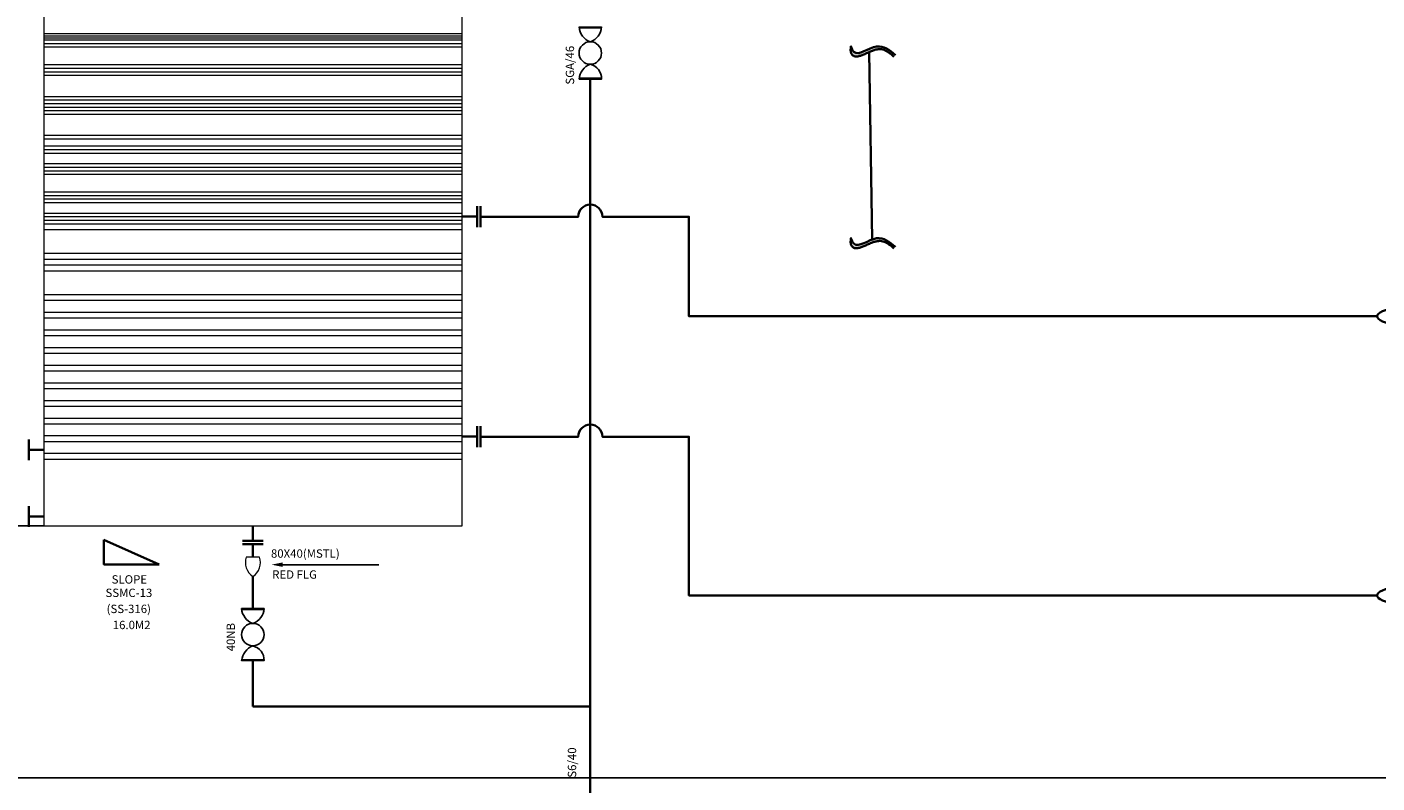
# Model space of a CAD drawing. Units: millimetres. Extents: x 353872 to 441597, y 126154 to 187356.
# Tile 23 of 28: x 399262 to 415084, y 157042 to 165906. Entities that reach past the tile are written whole.
import ezdxf

# ---------------------------------------------------------------- set-up
doc = ezdxf.new("R2010")
doc.units = ezdxf.units.MM
doc.linetypes.add('ACAD_ISO02W100', pattern=[15, 12, -3])
for name, color, linetype, lineweight in [('A-ANNO-DIMS', 2, 'Continuous', 18), ('P-ANNO-TEXT', 7, 'Continuous', 25), ('P-BNDY', 4, 'ACAD_ISO02W100', 25), ('P-INST-SIGN', 4, 'Continuous', 18), ('P-PIPE', 3, 'Continuous', 35), ('P-PIPE-FITT', 6, 'Continuous', 25), ('P-SYMB-PATT', 8, 'Continuous', 13), ('P-VALV', 2, 'Continuous', 25)]:
    doc.layers.add(name, color=color, linetype=linetype, lineweight=lineweight)
doc.layers.add('AC-UINT', color=2, linetype='Continuous')
doc.styles.get("Standard").update_dxf_attribs({"font": 'arial.ttf'})
doc.dimstyles.get("Standard").update_dxf_attribs({"dimtxt": 0.18, "dimasz": 0.18, "dimexe": 0.18, "dimexo": 0.0625, "dimgap": 0.09, "dimtad": 0, "dimtih": 1, "dimtoh": 1, "dimdec": 4, "dimzin": 0, "dimdsep": 46, "dimtxsty": 'Standard', "dimcen": 0.09, "dimadec": 0, "dimazin": 0, "dimtfac": 1, "dimtdec": 4, "dimtofl": 0, "dimtmove": 0, "dimatfit": 3, "dimfxl": 1, "dimtolj": 1, "dimtzin": 0, "dimarcsym": 0})

# ---------------------------------------------------------------- blocks, each defined once
blk = doc.blocks.new('DFSG')
at = {"layer": 'AC-UINT', "ltscale": 3}
blk.add_line((94.324, -27.16), (94.091, -27.16), dxfattribs=at)
blk.add_solid([(94.091, -27.121), (94.091, -27.199), (93.897, -27.16)], dxfattribs=at)
blk = doc.blocks.new('VALVE-L')
for points in [[(0, 9), (264, 9)], [(0, 0), (264, 0), (264, 3)]]:
    blk.add_lwpolyline(points)
for centre, radius, start, end in [((204, -19), 205, 110.6617, 174.7476), ((86, 2), 178, 359.5088, 75.082)]:
    blk.add_arc(centre, radius, start, end)
blk = doc.blocks.new('VALVE-N')
for points in [[(264, 173), (0, 173)], [(263, 164), (1, 164)]]:
    blk.add_lwpolyline(points)
for centre, radius, start, end in [((199, 188), 200, 184.2463, 250.3444), ((64, 189), 201, 289.8639, 355.5453)]:
    blk.add_arc(centre, radius, start, end)
blk = doc.blocks.new('VALVE-P')
blk.add_lwpolyline([(264, 173), (0, 173)])
for centre, radius, start, end in [((199, 188), 200, 184.2463, 250.3444), ((64, 189), 201, 289.8639, 355.5453)]:
    blk.add_arc(centre, radius, start, end)
blk = doc.blocks.new('*D34')
at = {"layer": 'A-ANNO-DIMS', "color": 0, "lineweight": -2, "transparency": 16777216}
for p, q in [((399457, 167930), (356736, 167930)), ((356737, 167930), (356737, 163994)), ((356737, 160058), (356737, 163994)), ((399457, 160058), (356736, 160058))]:
    blk.add_line(p, q, dxfattribs=at)
at = {"layer": 'A-ANNO-DIMS', "color": 0, "transparency": 16777216}
for points in [[(356737, 167930), (356737, 167930), (356737, 167930)], [(356737, 160058), (356737, 160058), (356737, 160058)]]:
    blk.add_solid(points, dxfattribs=at)
at = {"layer": 'Defpoints', "color": 0, "transparency": 16777216}
for p in [(399457, 167930), (356737, 160058), (399457, 160058)]:
    blk.add_point(p, dxfattribs=at)
at = {"layer": 'A-ANNO-DIMS', "color": 0, "transparency": 16777216, "insert": (356737, 163994), "char_height": 0.18, "attachment_point": 5}
blk.add_mtext('\\A1;7872', dxfattribs=at)

msp = doc.modelspace()

# ---------------------------------------------------------------- hatches: boundary and pattern name
at = {"layer": 'P-SYMB-PATT'}
h = msp.add_hatch(color=256, dxfattribs=at)
h.dxf.hatch_style = 1
edge = h.paths.add_edge_path()
edge.add_spline(control_points=[(408917.99, 165680.58), (408917.77, 165678.03), (408917.53, 165675.45), (408916.86, 165667.65), (408916.43, 165662.37), (408915.72, 165651.32), (408915.46, 165645.54), (408915.37, 165633.97), (408915.54, 165628.18), (408916.46, 165619.1), (408916.91, 165615.88), (408918.03, 165610.21), (408918.61, 165607.78), (408920.06, 165602.87), (408920.91, 165600.42), (408923.58, 165594.03), (408925.66, 165590.13), (408930.71, 165582.79), (408933.7, 165579.35), (408940.35, 165573.29), (408944.01, 165570.69), (408951.6, 165566.45), (408955.51, 165564.82), (408963.25, 165562.39), (408967.09, 165561.58), (408974.6, 165560.55), (408978.27, 165560.34), (408988.56, 165560.31), (408995, 165561), (409007.75, 165563.2), (409014.06, 165564.72), (409026.78, 165568.35), (409033.18, 165570.46), (409046.17, 165575.13), (409052.75, 165577.68), (409073.61, 165586.15), (409088.23, 165592.62), (409117.88, 165605.75), (409132.9, 165612.41), (409162.54, 165624.69), (409177.15, 165630.3), (409197.61, 165636.91), (409204.04, 165638.79), (409214.69, 165641.48), (409219.02, 165642.45), (409226.64, 165643.89), (409229.98, 165644.42), (409236.56, 165645.27), (409239.8, 165645.59), (409249.33, 165646.25), (409255.47, 165646.28), (409271.94, 165645.41), (409281.96, 165643.78), (409301.62, 165638.64), (409311.25, 165635.13), (409330.45, 165626.42), (409340.01, 165621.22), (409359.16, 165609.46), (409368.75, 165602.89), (409391.79, 165586.09), (409405.28, 165575.42), (409420.12, 165557.88)], knot_values=[0, 0, 0, 0, 1.45657696, 1.45657696, 4.36973087, 4.36973087, 7.5343006, 7.5343006, 10.69887033, 10.69887033, 12.40671205, 12.40671205, 13.63901259, 13.63901259, 14.87131314, 14.87131314, 16.90061252, 16.90061252, 18.92991189, 18.92991189, 20.95921127, 20.95921127, 22.98851065, 22.98851065, 25.01781003, 25.01781003, 27.04710941, 27.04710941, 30.82532254, 30.82532254, 34.60353567, 34.60353567, 38.38174881, 38.38174881, 42.15996194, 42.15996194, 50.18983557, 50.18983557, 58.21970919, 58.21970919, 66.24958282, 66.24958282, 70.07411996, 70.07411996, 72.8401263, 72.8401263, 75.12034604, 75.12034604, 77.40056578, 77.40056578, 81.96100526, 81.96100526, 89.95516575, 89.95516575, 97.94932623, 97.94932623, 105.94348671, 105.94348671, 113.9376472, 113.9376472, 125.00201057, 125.00201057, 125.00201057, 125.00201057], degree=3, periodic=0)
edge.add_line((409420.12, 165557.88), (409440.45, 165576.36))
edge.add_spline(control_points=[(409440.45, 165576.36), (409372.47, 165633.03), (409290.92, 165701.03), (409185.02, 165669.9), (409167.18, 165663.31)], knot_values=[65.29657048, 65.29657048, 65.29657048, 65.29657048, 118.21354525, 128.78520648, 128.78520648, 128.78520648, 128.78520648], degree=3, periodic=0)
edge.add_spline(control_points=[(409167.18, 165663.31), (409084.1, 165632.62), (408968.05, 165551.46), (408927.87, 165655.09), (408917.99, 165680.58)], knot_values=[0, 0, 0, 0, 49.23816608, 65.29657048, 65.29657048, 65.29657048, 65.29657048], degree=3, periodic=0)
h = msp.add_hatch(color=256, dxfattribs=at)
h.dxf.hatch_style = 1
edge = h.paths.add_edge_path()
edge.add_spline(control_points=[(408917.99, 163431.78), (408917.77, 163429.23), (408917.53, 163426.65), (408916.86, 163418.85), (408916.43, 163413.58), (408915.72, 163402.52), (408915.46, 163396.75), (408915.37, 163385.17), (408915.54, 163379.39), (408916.46, 163370.3), (408916.91, 163367.08), (408918.03, 163361.41), (408918.61, 163358.98), (408920.06, 163354.07), (408920.91, 163351.62), (408923.58, 163345.24), (408925.66, 163341.34), (408930.71, 163333.99), (408933.7, 163330.55), (408940.35, 163324.49), (408944.01, 163321.89), (408951.6, 163317.66), (408955.51, 163316.02), (408963.25, 163313.59), (408967.09, 163312.78), (408974.6, 163311.76), (408978.27, 163311.54), (408988.56, 163311.52), (408995, 163312.21), (409007.75, 163314.4), (409014.06, 163315.92), (409026.78, 163319.55), (409033.18, 163321.66), (409046.17, 163326.33), (409052.75, 163328.88), (409073.61, 163337.35), (409088.23, 163343.82), (409117.88, 163356.95), (409132.9, 163363.62), (409162.54, 163375.9), (409177.15, 163381.51), (409197.61, 163388.11), (409204.04, 163389.99), (409214.69, 163392.69), (409219.02, 163393.65), (409226.64, 163395.1), (409229.98, 163395.63), (409236.56, 163396.48), (409239.8, 163396.79), (409249.33, 163397.45), (409255.47, 163397.48), (409271.94, 163396.61), (409281.96, 163394.98), (409301.62, 163389.84), (409311.25, 163386.33), (409330.45, 163377.62), (409340.01, 163372.43), (409359.16, 163360.66), (409368.75, 163354.09), (409391.79, 163337.29), (409405.28, 163326.62), (409420.12, 163309.08)], knot_values=[0, 0, 0, 0, 1.45657696, 1.45657696, 4.36973087, 4.36973087, 7.5343006, 7.5343006, 10.69887033, 10.69887033, 12.40671205, 12.40671205, 13.63901259, 13.63901259, 14.87131314, 14.87131314, 16.90061252, 16.90061252, 18.92991189, 18.92991189, 20.95921127, 20.95921127, 22.98851065, 22.98851065, 25.01781003, 25.01781003, 27.04710941, 27.04710941, 30.82532254, 30.82532254, 34.60353567, 34.60353567, 38.38174881, 38.38174881, 42.15996194, 42.15996194, 50.18983557, 50.18983557, 58.21970919, 58.21970919, 66.24958282, 66.24958282, 70.07411996, 70.07411996, 72.8401263, 72.8401263, 75.12034604, 75.12034604, 77.40056578, 77.40056578, 81.96100526, 81.96100526, 89.95516575, 89.95516575, 97.94932623, 97.94932623, 105.94348671, 105.94348671, 113.9376472, 113.9376472, 125.00201057, 125.00201057, 125.00201057, 125.00201057], degree=3, periodic=0)
edge.add_line((409420.12, 163309.08), (409440.45, 163327.56))
edge.add_spline(control_points=[(409440.45, 163327.56), (409372.47, 163384.24), (409290.92, 163452.23), (409185.02, 163421.1), (409167.18, 163414.52)], knot_values=[65.29657048, 65.29657048, 65.29657048, 65.29657048, 118.21354525, 128.78520648, 128.78520648, 128.78520648, 128.78520648], degree=3, periodic=0)
edge.add_spline(control_points=[(409167.18, 163414.52), (409084.1, 163383.82), (408968.05, 163302.67), (408927.87, 163406.3), (408917.99, 163431.78)], knot_values=[0, 0, 0, 0, 49.23816608, 65.29657048, 65.29657048, 65.29657048, 65.29657048], degree=3, periodic=0)

# ---------------------------------------------------------------- linework, layer by layer
at = {"layer": 'P-BNDY'}
for p, q in [((402415.77, 159602.24), (403386.8, 159602.24)), ((436591, 157104.68), (386532.91, 157104.68))]:
    msp.add_line(p, q, dxfattribs=at)
at = {"layer": 'P-INST-SIGN'}
for p, q in [((399457.15, 165828.71), (404363.17, 165828.71)), ((399457.15, 165804.32), (404363.17, 165804.32)), ((399457.15, 165779.93), (404363.17, 165779.93)), ((399457.15, 165755.54), (404363.17, 165755.54)), ((399457.15, 165714.08), (404363.17, 165714.08)), ((399457.15, 165672.62), (404363.17, 165672.62)), ((399457.15, 165465.32), (404363.17, 165465.32)), ((399457.15, 165423.86), (404363.17, 165423.86)), ((399457.15, 165382.4), (404363.17, 165382.4)), ((399457.15, 165340.94), (404363.17, 165340.94)), ((399457.15, 165092.18), (404363.17, 165092.18)), ((399457.15, 165050.72), (404363.17, 165050.72)), ((399457.15, 165009.26), (404363.17, 165009.26)), ((399457.15, 164967.8), (404363.17, 164967.8)), ((399457.15, 164926.34), (404363.17, 164926.34)), ((399457.15, 164884.88), (404363.17, 164884.88)), ((399457.15, 164636.12), (404363.17, 164636.12)), ((399457.15, 164594.66), (404363.17, 164594.66)), ((399457.15, 164511.74), (404363.17, 164511.74)), ((399457.15, 164470.28), (404363.17, 164470.28)), ((399457.15, 164428.82), (404363.17, 164428.82)), ((399457.15, 164304.44), (404363.17, 164304.44)), ((399457.15, 164262.98), (404363.17, 164262.98)), ((399457.15, 164221.52), (404363.17, 164221.52)), ((399457.15, 164180.06), (404363.17, 164180.06)), ((399457.15, 163972.76), (404363.17, 163972.76)), ((399457.15, 163931.3), (404363.17, 163931.3)), ((399457.15, 163889.84), (404363.17, 163889.84)), ((399457.15, 163848.38), (404363.17, 163848.38)), ((399457.15, 163724), (404363.17, 163724)), ((399457.15, 163682.54), (404363.17, 163682.54)), ((399457.15, 163641.08), (404363.17, 163641.08)), ((399457.15, 163599.62), (404363.17, 163599.62)), ((399457.15, 163530.6), (404363.17, 163530.6)), ((399457.15, 163254.51), (404363.17, 163254.51)), ((399457.15, 163185.49), (404363.17, 163185.49)), ((399457.15, 163116.46), (404363.17, 163116.46)), ((399457.15, 163047.44), (404363.17, 163047.44)), ((399457.15, 162771.35), (404363.17, 162771.35)), ((399457.15, 162702.33), (404363.17, 162702.33)), ((399457.15, 162564.29), (404363.17, 162564.29)), ((399457.15, 162495.26), (404363.17, 162495.26)), ((399457.15, 162495.26), (404363.17, 162495.26)), ((399457.15, 162357.22), (404363.17, 162357.22)), ((399457.15, 162288.2), (404363.17, 162288.2)), ((399457.15, 162150.15), (404363.17, 162150.15)), ((399457.15, 162081.13), (404363.17, 162081.13)), ((399457.15, 161943.09), (404363.17, 161943.09)), ((399457.15, 161874.06), (404363.17, 161874.06)), ((399457.15, 161736.02), (404363.17, 161736.02)), ((399457.15, 161667), (404363.17, 161667)), ((399457.15, 161528.95), (404363.17, 161528.95)), ((399457.15, 161459.93), (404363.17, 161459.93)), ((399457.15, 161321.88), (404363.17, 161321.88)), ((399457.15, 161252.86), (404363.17, 161252.86)), ((399457.15, 161114.82), (404363.17, 161114.82)), ((399457.15, 161045.8), (404363.17, 161045.8)), ((399457.15, 160907.75), (404363.17, 160907.75)), ((399457.15, 160838.73), (404363.17, 160838.73))]:
    msp.add_line(p, q, dxfattribs=at)
msp.add_lwpolyline([(404363.17, 167929.97), (399457.15, 167929.97), (399457.15, 160058.19), (404363.17, 160058.19)], close=True, dxfattribs=at)
msp.add_lwpolyline([(401986.75, 159691.83), (401831.53, 159691.83)], dxfattribs=at)
for centre, radius, start, end in [((402025.02, 159629.39), 203.32, 162.115929, 235.252176), ((401800.51, 159626.94), 197.22, 303.422212, 19.209682)]:
    msp.add_arc(centre, radius, start, end, dxfattribs=at)
at = {"layer": 'P-PIPE'}
for p, q in [((409167.18, 163414.52), (409133.01, 165612.33)), ((405863.95, 165296.06), (405863.95, 157658.81)), ((404538.96, 163803.9), (404538.96, 163559.14)), ((404578.12, 163803.9), (404578.12, 163559.14)), ((404363.17, 163682.54), (404538.96, 163682.54)), ((404363.17, 161103.43), (404538.96, 161103.43)), ((404538.96, 161224.78), (404538.96, 160980.02)), ((404578.12, 161224.78), (404578.12, 160980.02)), ((399281.36, 160826.46), (399281.36, 161071.22)), ((399457.15, 160947.82), (399281.36, 160947.82)), ((399281.36, 160044.44), (399281.36, 160289.2)), ((399457.15, 160165.8), (399281.36, 160165.8)), ((401910.16, 160058.19), (401910.16, 159882.39)), ((400163.76, 159891.76), (400810.39, 159604.6)), ((402031.52, 159882.39), (401786.76, 159882.39)), ((402031.52, 159843.23), (401786.76, 159843.23)), ((401909.14, 159843.23), (401909.14, 159691.83)), ((401909.14, 159462.33), (401909.14, 159078.04)), ((401909.15, 158476.97), (401909.08, 157939.91)), ((401909.08, 157939.91), (405863.95, 157939.91)), ((405863.95, 157658.81), (405863.95, 156248.03))]:
    msp.add_line(p, q, dxfattribs=at)
for points in [[(415084.48, 162514.19), (407019.22, 162514.19), (407019.22, 163681.52), (406832.69, 163681.52), (406005.7, 163681.52, 1), (405722.2, 163681.52), (404578.12, 163681.52)], [(415084.48, 159241.9), (407019.22, 159241.9), (407019.22, 161102.4), (406005.7, 161102.4, 1), (405722.2, 161102.4), (404578.12, 161102.4)]]:
    msp.add_lwpolyline(points, format="xyb", dxfattribs=at)
msp.add_lwpolyline([(400163.76, 159891.76), (400163.76, 159604.6), (400810.39, 159604.6)], dxfattribs=at)
for centre in [(415913.9, 162514.19), (415913.9, 162514.19), (415913.9, 159241.9), (415913.9, 159241.9)]:
    msp.add_ellipse(centre, major_axis=(829.42, 0), ratio=0.18269243, dxfattribs=at)
for points in [[(409440.45, 165576.36), (409372.47, 165633.03), (409227.68, 165753.76), (408974.55, 165534.69), (408927.87, 165655.09), (408917.99, 165680.58), (408917.77, 165678.03), (408917.53, 165675.45), (408916.86, 165667.65), (408916.43, 165662.37), (408915.72, 165651.32), (408915.46, 165645.54), (408915.37, 165633.97), (408915.54, 165628.18), (408916.46, 165619.1), (408916.91, 165615.88), (408918.03, 165610.21), (408918.61, 165607.78), (408920.06, 165602.87), (408920.91, 165600.42), (408923.58, 165594.03), (408925.66, 165590.13), (408930.71, 165582.79), (408933.7, 165579.35), (408940.35, 165573.29), (408944.01, 165570.69), (408951.6, 165566.45), (408955.51, 165564.82), (408963.25, 165562.39), (408967.09, 165561.58), (408974.6, 165560.55), (408978.27, 165560.34), (408988.56, 165560.31), (408995, 165561), (409007.75, 165563.2), (409014.06, 165564.72), (409026.78, 165568.35), (409033.18, 165570.46), (409046.17, 165575.13), (409052.75, 165577.68), (409073.61, 165586.15), (409088.23, 165592.62), (409117.88, 165605.75), (409132.9, 165612.41), (409162.54, 165624.69), (409177.15, 165630.3), (409197.61, 165636.91), (409204.04, 165638.79), (409214.69, 165641.48), (409219.02, 165642.45), (409226.64, 165643.89), (409229.98, 165644.42), (409236.56, 165645.27), (409239.8, 165645.59), (409249.33, 165646.25), (409255.47, 165646.28), (409271.94, 165645.41), (409281.96, 165643.78), (409301.62, 165638.64), (409311.25, 165635.13), (409330.45, 165626.42), (409340.01, 165621.22), (409359.16, 165609.46), (409368.75, 165602.89), (409391.79, 165586.09), (409405.28, 165575.42), (409420.12, 165557.88)], [(409440.45, 163327.56), (409372.47, 163384.24), (409227.68, 163504.96), (408974.55, 163285.89), (408927.87, 163406.3), (408917.99, 163431.78), (408917.77, 163429.23), (408917.53, 163426.65), (408916.86, 163418.85), (408916.43, 163413.58), (408915.72, 163402.52), (408915.46, 163396.75), (408915.37, 163385.17), (408915.54, 163379.39), (408916.46, 163370.3), (408916.91, 163367.08), (408918.03, 163361.41), (408918.61, 163358.98), (408920.06, 163354.07), (408920.91, 163351.62), (408923.58, 163345.24), (408925.66, 163341.34), (408930.71, 163333.99), (408933.7, 163330.55), (408940.35, 163324.49), (408944.01, 163321.89), (408951.6, 163317.66), (408955.51, 163316.02), (408963.25, 163313.59), (408967.09, 163312.78), (408974.6, 163311.76), (408978.27, 163311.54), (408988.56, 163311.52), (408995, 163312.21), (409007.75, 163314.4), (409014.06, 163315.92), (409026.78, 163319.55), (409033.18, 163321.66), (409046.17, 163326.33), (409052.75, 163328.88), (409073.61, 163337.35), (409088.23, 163343.82), (409117.88, 163356.95), (409132.9, 163363.62), (409162.54, 163375.9), (409177.15, 163381.51), (409197.61, 163388.11), (409204.04, 163389.99), (409214.69, 163392.69), (409219.02, 163393.65), (409226.64, 163395.1), (409229.98, 163395.63), (409236.56, 163396.48), (409239.8, 163396.79), (409249.33, 163397.45), (409255.47, 163397.48), (409271.94, 163396.61), (409281.96, 163394.98), (409301.62, 163389.84), (409311.25, 163386.33), (409330.45, 163377.62), (409340.01, 163372.43), (409359.16, 163360.66), (409368.75, 163354.09), (409391.79, 163337.29), (409405.28, 163326.62), (409420.12, 163309.08)]]:
    msp.add_open_spline(points, degree=3, knots=[0, 0, 0, 0, 178.42679837, 380.09509195, 434.24122741, 434.24122741, 434.24122741, 435.69780436, 435.69780436, 438.61095828, 438.61095828, 441.775528, 441.775528, 444.94009773, 444.94009773, 446.64793946, 446.64793946, 447.88024, 447.88024, 449.11254054, 449.11254054, 451.14183992, 451.14183992, 453.1711393, 453.1711393, 455.20043868, 455.20043868, 457.22973806, 457.22973806, 459.25903744, 459.25903744, 461.28833682, 461.28833682, 465.06654995, 465.06654995, 468.84476308, 468.84476308, 472.62297621, 472.62297621, 476.40118935, 476.40118935, 484.43106297, 484.43106297, 492.4609366, 492.4609366, 500.49081023, 500.49081023, 504.31534737, 504.31534737, 507.0813537, 507.0813537, 509.36157345, 509.36157345, 511.64179319, 511.64179319, 516.20223267, 516.20223267, 524.19639315, 524.19639315, 532.19055364, 532.19055364, 540.18471412, 540.18471412, 548.1788746, 548.1788746, 559.24323797, 559.24323797, 559.24323797, 559.24323797], dxfattribs=at)
at = {"layer": 'P-VALV'}
msp.add_lwpolyline([(405994.93, 165897.12), (405732.94, 165897.12)], dxfattribs=at)
for centre in [(405863.95, 165601.12), (401909.15, 158782.04)]:
    msp.add_circle(centre, 131.9, dxfattribs=at)

# ---------------------------------------------------------------- block references
at = {"layer": 'P-PIPE-FITT', "xscale": 677.5688707767378, "yscale": 677.5688707767378, "zscale": 677.5688707767378}
msp.add_blockref('DFSG', (338504.98, 178005.09), dxfattribs=at)
at = {"layer": 'P-VALV'}
for name, p in [('VALVE-P', (405732.05, 165733.02)), ('VALVE-L', (405732.05, 165296.06)), ('VALVE-N', (401777.26, 158913.93)), ('VALVE-L', (401777.26, 158476.97))]:
    msp.add_blockref(name, p, dxfattribs=at)

# ---------------------------------------------------------------- texts
at = {"layer": 'P-ANNO-TEXT'}
for s, p in [('SGA/46', (405674.28, 165230.95)), ('40NB', (401699.22, 158585.96)), ('S6/40', (405698.53, 157104.68))]:
    msp.add_text(s, height=98.09, rotation=90, dxfattribs=at).set_placement(p)
for s, height, p in [('80X40(MSTL)', 98.0901, (402121.07, 159683.83)), ('RED FLG', 98.09, (402135.91, 159437.71)), ('SLOPE', 98.09, (400253.57, 159380.26)), ('SSMC-13', 98.09, (400181.72, 159223.23)), ('(SS-316)', 98.09, (400195.19, 159034.78)), ('16.0M2', 98.09, (400267.04, 158846.33))]:
    msp.add_text(s, height=height, dxfattribs=at).set_placement(p)

# ---------------------------------------------------------------- dimensions: what is measured, and where the dimension line sits
at = {"layer": 'A-ANNO-DIMS'}
dim = msp.add_linear_dim(base=(356736.55, 160058.19), p1=(399457.15, 167929.97), p2=(399457.15, 160058.19), angle=90, dimstyle='Standard', override={"dimdec": 0, "dimlfac": 1, "dimrnd": 0, "dimzin": 0, "dimdsep": 46, "dimlunit": 2}, dxfattribs=at)
dim.commit()
dim.dimension.update_dxf_attribs({"geometry": '*D34', "text_midpoint": (356736.55, 163994.08)})

doc.saveas('drawing.dxf')
